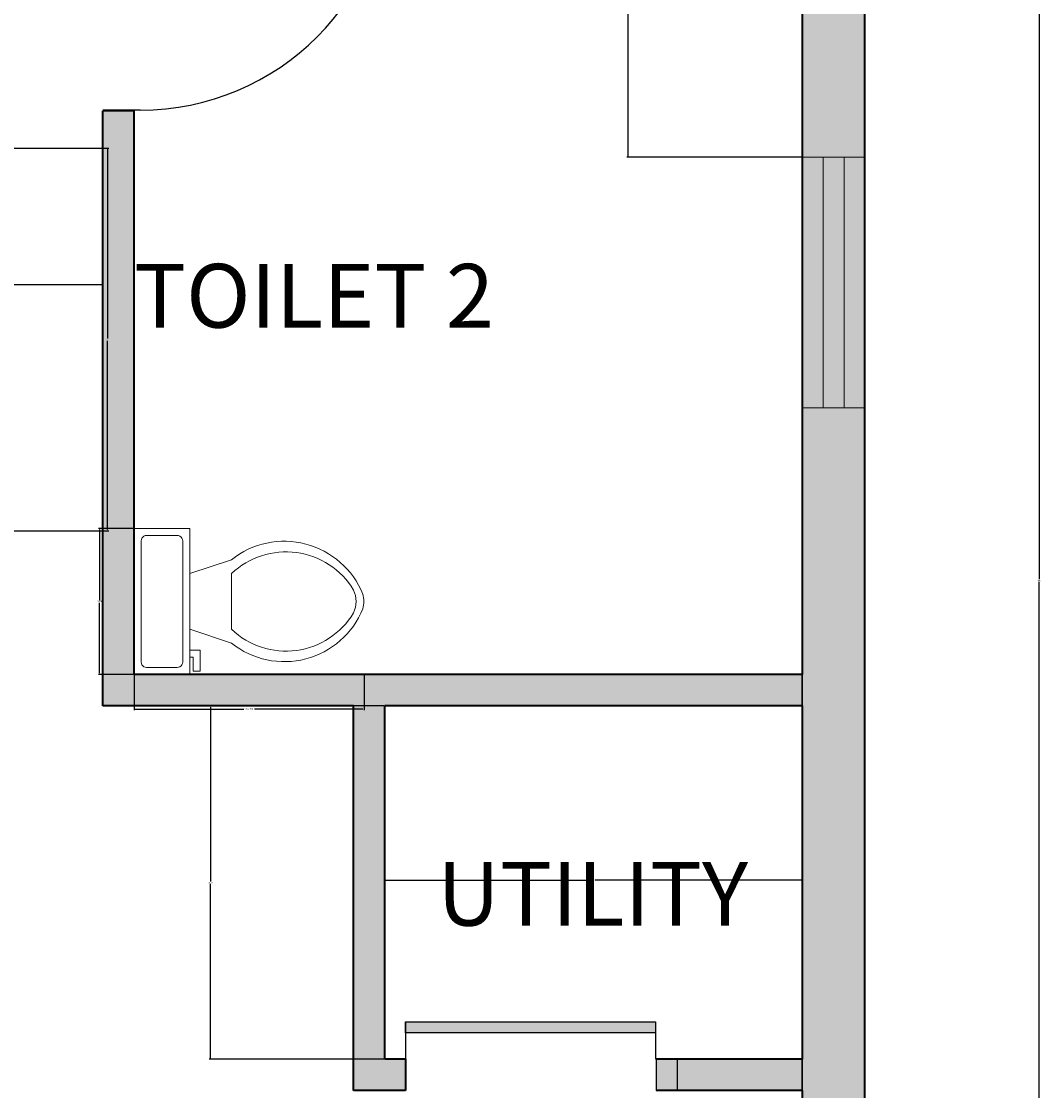
# Model space of a CAD drawing. Units: inches. Extents: x 1434 to 1845, y 1483 to 2014.
# Tile 8 of 11: x 1698 to 1845, y 1675 to 1829. Entities that reach past the tile are written whole.
import ezdxf

# ---------------------------------------------------------------- set-up
doc = ezdxf.new("R2010")
doc.units = ezdxf.units.IN
for name, color, linetype, lineweight in [('A-ANNO-DIMS', 2, 'Continuous', 18), ('A-AREA-IDEN', 7, 'Continuous', 25), ('A-DOOR', 3, 'Continuous', 25), ('A-FLOR-FIXT', 8, 'Continuous', 18), ('A-GLAZ', 4, 'Continuous', 18), ('A-GLAZ-PATT', 9, 'Continuous', 13), ('A-WALL', 7, 'Continuous', 35), ('A-WALL-PATT', 8, 'Continuous', 13)]:
    doc.layers.add(name, color=color, linetype=linetype, lineweight=lineweight)
doc.layers.add('A-DOOR-PATT', color=39, linetype='Continuous', lineweight=13, true_color=0x58382b)
doc.styles.get("Standard").update_dxf_attribs({"font": 'arial.ttf'})
doc.dimstyles.get("Standard").update_dxf_attribs({"dimtxt": 0.18, "dimasz": 0.18, "dimexe": 0.18, "dimexo": 0.0625, "dimgap": 0.09, "dimtad": 0, "dimtih": 1, "dimtoh": 1, "dimdec": 4, "dimzin": 0, "dimdsep": 46, "dimtxsty": 'Standard', "dimcen": 0.09, "dimadec": 0, "dimazin": 0, "dimtfac": 1, "dimtdec": 4, "dimtofl": 0, "dimtmove": 0, "dimatfit": 3, "dimfxl": 1, "dimtolj": 1, "dimtzin": 0, "dimarcsym": 0})

# ---------------------------------------------------------------- blocks, each defined once
blk = doc.blocks.new('*U3')
for p, q in [((0, 0), (0, -6)), ((40, 0), (40, -6))]:
    blk.add_line(p, q)
blk.add_lwpolyline([(0, 0), (0, 40), (1.75, 40), (1.75, 0)], close=True)
blk.add_arc((0, 0), 40, 0, 90)
blk = doc.blocks.new('*U5')
for p, q in [((0, 0), (0, -6)), ((40, 0), (40, -6))]:
    blk.add_line(p, q)
blk.add_lwpolyline([(0, 0), (40, 0), (40, -1.75), (0, -1.75)], close=True)
blk = doc.blocks.new('Toilet - top')
for p, q in [((9.5, -6), (9.5, -2)), ((-10, -8.5), (-8, -8.5)), ((-10, -9.5), (-10, -8.5)), ((-8, -8.5), (-8, -8)), ((-7, -8), (-7, -9.5)), ((-4, -8), (-6, -14)), ((4, -8), (6, -14)), ((-7, -9.5), (-10, -9.5)), ((4, -14), (-4, -14))]:
    blk.add_line(p, q)
blk.add_lwpolyline([(10.5, -8), (10.5, 0), (-10.5, 0), (-10.5, -8)], close=True)
for points in [[(8.5, -1), (-8.5, -1)], [(-9.5, -2), (-9.5, -6)], [(-8.5, -7), (8.5, -7)]]:
    blk.add_lwpolyline(points)
for centre, radius, start, end in [((-8.62, -1.88), 0.884, 81.8699, 188.1301), ((8.62, -1.88), 0.884, 351.8699, 98.1301), ((-8.62, -6.12), 0.884, 171.8699, 278.1301), ((8.62, -6.12), 0.884, 261.8699, 8.1301), ((3.52, -21.58), 12.17, 141.4691, 247.9714), ((4.2, -21.82), 11.33, 136.3677, 238.9468), ((-3.52, -21.58), 12.17, 292.0284, 38.5307), ((-4.2, -21.82), 11.33, 301.053, 43.6321), ((0, -27.88), 4, 245.7318, 294.2682), ((0, -29), 4, 254.8605, 285.1395)]:
    blk.add_arc(centre, radius, start, end)
blk = doc.blocks.new('WIN-36IN-9IN')
for p, q in [((3, 36), (3, 0)), ((6, 36), (6, 0))]:
    blk.add_line(p, q)
blk.add_lwpolyline([(9, 0), (9, 36), (0, 36), (0, 0)], close=True)
blk = doc.blocks.new('*D36')
at = {"layer": 'A-ANNO-DIMS', "color": 0, "lineweight": -2, "transparency": 16777216}
for p, q in [((1714.47, 1734.79), (1714.47, 1729.72)), ((1747.52, 1734.79), (1747.52, 1729.72)), ((1714.65, 1729.9), (1730.22, 1729.9)), ((1747.34, 1729.9), (1731.77, 1729.9))]:
    blk.add_line(p, q, dxfattribs=at)
at = {"layer": 'A-ANNO-DIMS', "color": 0, "transparency": 16777216}
for points in [[(1714.65, 1729.93), (1714.65, 1729.87), (1714.47, 1729.9)], [(1747.34, 1729.93), (1747.34, 1729.87), (1747.52, 1729.9)]]:
    blk.add_solid(points, dxfattribs=at)
at = {"layer": 'Defpoints', "color": 0, "transparency": 16777216}
for p in [(1714.47, 1734.86), (1747.52, 1734.86), (1714.47, 1729.9)]:
    blk.add_point(p, dxfattribs=at)
at = {"layer": 'A-ANNO-DIMS', "color": 0, "transparency": 16777216, "insert": (1731, 1729.9), "char_height": 0.18, "attachment_point": 5}
blk.add_mtext('\\A1;WC 33 TYP.', dxfattribs=at)
blk = doc.blocks.new('*D37')
at = {"layer": 'A-ANNO-DIMS', "color": 0, "lineweight": -2, "transparency": 16777216}
for p, q in [((1714.41, 1755.86), (1709.34, 1755.86)), ((1709.52, 1755.68), (1709.52, 1745.54)), ((1709.52, 1735.04), (1709.52, 1745.17)), ((1714.41, 1734.86), (1709.34, 1734.86))]:
    blk.add_line(p, q, dxfattribs=at)
at = {"layer": 'A-ANNO-DIMS', "color": 0, "transparency": 16777216}
for points in [[(1709.49, 1755.68), (1709.55, 1755.68), (1709.52, 1755.86)], [(1709.49, 1735.04), (1709.55, 1735.04), (1709.52, 1734.86)]]:
    blk.add_solid(points, dxfattribs=at)
at = {"layer": 'Defpoints', "color": 0, "transparency": 16777216}
for p in [(1709.52, 1755.86), (1714.47, 1755.86), (1714.47, 1734.86)]:
    blk.add_point(p, dxfattribs=at)
at = {"layer": 'A-ANNO-DIMS', "color": 0, "transparency": 16777216, "insert": (1709.52, 1745.36), "char_height": 0.18, "attachment_point": 5}
blk.add_mtext('\\A1;21 TYP.', dxfattribs=at)
blk = doc.blocks.new('*D43')
at = {"layer": 'A-ANNO-DIMS', "color": 0, "lineweight": -2, "transparency": 16777216}
for p, q in [((1697.08, 1810.5), (1710.85, 1810.5)), ((1710.67, 1810.32), (1710.67, 1783.19)), ((1710.67, 1755.68), (1710.67, 1782.82)), ((1697.08, 1755.5), (1710.85, 1755.5))]:
    blk.add_line(p, q, dxfattribs=at)
at = {"layer": 'A-ANNO-DIMS', "color": 0, "transparency": 16777216}
for points in [[(1710.64, 1810.32), (1710.7, 1810.32), (1710.67, 1810.5)], [(1710.64, 1755.68), (1710.7, 1755.68), (1710.67, 1755.5)]]:
    blk.add_solid(points, dxfattribs=at)
at = {"layer": 'Defpoints', "color": 0, "transparency": 16777216}
for p in [(1697.02, 1810.5), (1710.67, 1810.5), (1697.02, 1755.5)]:
    blk.add_point(p, dxfattribs=at)
at = {"layer": 'A-ANNO-DIMS', "color": 0, "transparency": 16777216, "insert": (1710.67, 1783), "char_height": 0.18, "attachment_point": 5}
blk.add_mtext('\\A1;55', dxfattribs=at)
blk = doc.blocks.new('*D55')
at = {"layer": 'A-ANNO-DIMS', "color": 0, "lineweight": -2, "transparency": 16777216}
for p, q in [((1819.54, 1988.36), (1844.68, 1988.36)), ((1844.5, 1988.18), (1844.5, 1748.54)), ((1844.5, 1508.54), (1844.5, 1748.17)), ((1819.54, 1508.36), (1844.68, 1508.36))]:
    blk.add_line(p, q, dxfattribs=at)
at = {"layer": 'A-ANNO-DIMS', "color": 0, "transparency": 16777216}
for points in [[(1844.47, 1988.18), (1844.53, 1988.18), (1844.5, 1988.36)], [(1844.47, 1508.54), (1844.53, 1508.54), (1844.5, 1508.36)]]:
    blk.add_solid(points, dxfattribs=at)
at = {"layer": 'Defpoints', "color": 0, "transparency": 16777216}
for p in [(1819.47, 1988.36), (1844.5, 1988.36), (1819.47, 1508.36)]:
    blk.add_point(p, dxfattribs=at)
at = {"layer": 'A-ANNO-DIMS', "color": 0, "transparency": 16777216, "insert": (1844.5, 1748.36), "char_height": 0.18, "attachment_point": 5}
blk.add_mtext('\\A1;480', dxfattribs=at)
blk = doc.blocks.new('*D58')
at = {"layer": 'A-ANNO-DIMS', "color": 0, "lineweight": -2, "transparency": 16777216}
for p, q in [((1670.97, 1974.79), (1670.97, 1483.15)), ((1810.47, 1974.79), (1810.47, 1483.15)), ((1671.15, 1483.33), (1740.34, 1483.33)), ((1810.29, 1483.33), (1741.11, 1483.33))]:
    blk.add_line(p, q, dxfattribs=at)
at = {"layer": 'A-ANNO-DIMS', "color": 0, "transparency": 16777216}
for points in [[(1671.15, 1483.36), (1671.15, 1483.3), (1670.97, 1483.33)], [(1810.29, 1483.36), (1810.29, 1483.3), (1810.47, 1483.33)]]:
    blk.add_solid(points, dxfattribs=at)
at = {"layer": 'Defpoints', "color": 0, "transparency": 16777216}
for p in [(1670.97, 1974.86), (1810.47, 1974.86), (1810.47, 1483.33)]:
    blk.add_point(p, dxfattribs=at)
at = {"layer": 'A-ANNO-DIMS', "color": 0, "transparency": 16777216, "insert": (1740.72, 1483.33), "char_height": 0.18, "attachment_point": 5}
blk.add_mtext('\\A1;139.5', dxfattribs=at)
blk = doc.blocks.new('*D62')
at = {"layer": 'A-ANNO-DIMS', "color": 0, "lineweight": -2, "transparency": 16777216}
for p, q in [((1573.47, 1815.79), (1573.47, 1790.65)), ((1709.97, 1815.79), (1709.97, 1790.65)), ((1573.65, 1790.83), (1641.34, 1790.83)), ((1709.79, 1790.83), (1642.11, 1790.83))]:
    blk.add_line(p, q, dxfattribs=at)
at = {"layer": 'A-ANNO-DIMS', "color": 0, "transparency": 16777216}
for points in [[(1573.65, 1790.86), (1573.65, 1790.8), (1573.47, 1790.83)], [(1709.79, 1790.86), (1709.79, 1790.8), (1709.97, 1790.83)]]:
    blk.add_solid(points, dxfattribs=at)
at = {"layer": 'Defpoints', "color": 0, "transparency": 16777216}
for p in [(1573.47, 1815.86), (1709.97, 1815.86), (1573.47, 1790.83)]:
    blk.add_point(p, dxfattribs=at)
at = {"layer": 'A-ANNO-DIMS', "color": 0, "transparency": 16777216, "insert": (1641.72, 1790.83), "char_height": 0.18, "attachment_point": 5}
blk.add_mtext('\\A1;136.5', dxfattribs=at)
blk = doc.blocks.new('*D67')
at = {"layer": 'A-ANNO-DIMS', "color": 0, "lineweight": -2, "transparency": 16777216}
for p, q in [((1694.97, 1517.42), (1694.97, 2013.56)), ((1695.15, 2013.38), (1752.34, 2013.38)), ((1810.29, 2013.38), (1753.11, 2013.38)), ((1810.47, 1517.42), (1810.47, 2013.56))]:
    blk.add_line(p, q, dxfattribs=at)
at = {"layer": 'A-ANNO-DIMS', "color": 0, "transparency": 16777216}
for points in [[(1695.15, 2013.41), (1695.15, 2013.35), (1694.97, 2013.38)], [(1810.29, 2013.41), (1810.29, 2013.35), (1810.47, 2013.38)]]:
    blk.add_solid(points, dxfattribs=at)
at = {"layer": 'Defpoints', "color": 0, "transparency": 16777216}
for p in [(1810.47, 2013.38), (1694.97, 1517.36), (1810.47, 1517.36)]:
    blk.add_point(p, dxfattribs=at)
at = {"layer": 'A-ANNO-DIMS', "color": 0, "transparency": 16777216, "insert": (1752.72, 2013.38), "char_height": 0.18, "attachment_point": 5}
blk.add_mtext('\\A1;115.5', dxfattribs=at)
blk = doc.blocks.new('*D68')
at = {"layer": 'A-ANNO-DIMS', "color": 0, "lineweight": -2, "transparency": 16777216}
for p, q in [((1750.47, 1730.29), (1750.47, 1705.15)), ((1810.47, 1730.29), (1810.47, 1705.15)), ((1750.65, 1705.33), (1780.26, 1705.33)), ((1810.29, 1705.33), (1780.69, 1705.33))]:
    blk.add_line(p, q, dxfattribs=at)
at = {"layer": 'A-ANNO-DIMS', "color": 0, "transparency": 16777216}
for points in [[(1750.65, 1705.36), (1750.65, 1705.3), (1750.47, 1705.33)], [(1810.29, 1705.36), (1810.29, 1705.3), (1810.47, 1705.33)]]:
    blk.add_solid(points, dxfattribs=at)
at = {"layer": 'Defpoints', "color": 0, "transparency": 16777216}
for p in [(1750.47, 1730.36), (1810.47, 1730.36), (1750.47, 1705.33)]:
    blk.add_point(p, dxfattribs=at)
at = {"layer": 'A-ANNO-DIMS', "color": 0, "transparency": 16777216, "insert": (1780.47, 1705.33), "char_height": 0.18, "attachment_point": 5}
blk.add_mtext('\\A1;60', dxfattribs=at)
blk = doc.blocks.new('*D69')
at = {"layer": 'A-ANNO-DIMS', "color": 0, "lineweight": -2, "transparency": 16777216}
for p, q in [((1750.41, 1730.36), (1725.27, 1730.36)), ((1725.45, 1730.18), (1725.45, 1705.15)), ((1725.45, 1679.76), (1725.45, 1704.79)), ((1750.41, 1679.58), (1725.27, 1679.58))]:
    blk.add_line(p, q, dxfattribs=at)
at = {"layer": 'A-ANNO-DIMS', "color": 0, "transparency": 16777216}
for points in [[(1725.42, 1730.18), (1725.48, 1730.18), (1725.45, 1730.36)], [(1725.42, 1679.76), (1725.48, 1679.76), (1725.45, 1679.58)]]:
    blk.add_solid(points, dxfattribs=at)
at = {"layer": 'Defpoints', "color": 0, "transparency": 16777216}
for p in [(1725.45, 1730.36), (1750.47, 1730.36), (1750.47, 1679.58)]:
    blk.add_point(p, dxfattribs=at)
at = {"layer": 'A-ANNO-DIMS', "color": 0, "transparency": 16777216, "insert": (1725.45, 1704.97), "char_height": 0.18, "attachment_point": 5}
blk.add_mtext('\\A1;50.77', dxfattribs=at)
blk = doc.blocks.new('*D79')
at = {"layer": 'A-ANNO-DIMS', "color": 0, "lineweight": -2, "transparency": 16777216}
for p, q in [((1810.41, 1854.86), (1785.27, 1854.86)), ((1785.45, 1854.68), (1785.45, 1832.19)), ((1785.45, 1809.35), (1785.45, 1831.83)), ((1810.41, 1809.17), (1785.27, 1809.17))]:
    blk.add_line(p, q, dxfattribs=at)
at = {"layer": 'A-ANNO-DIMS', "color": 0, "transparency": 16777216}
for points in [[(1785.42, 1854.68), (1785.48, 1854.68), (1785.45, 1854.86)], [(1785.42, 1809.35), (1785.48, 1809.35), (1785.45, 1809.17)]]:
    blk.add_solid(points, dxfattribs=at)
at = {"layer": 'Defpoints', "color": 0, "transparency": 16777216}
for p in [(1785.45, 1854.86), (1810.47, 1854.86), (1810.47, 1809.17)]:
    blk.add_point(p, dxfattribs=at)
at = {"layer": 'A-ANNO-DIMS', "color": 0, "transparency": 16777216, "insert": (1785.45, 1832.01), "char_height": 0.18, "attachment_point": 5}
blk.add_mtext('\\A1;45.69', dxfattribs=at)

msp = doc.modelspace()

# ---------------------------------------------------------------- hatches: boundary and pattern name
at = {"layer": 'A-DOOR-PATT'}
h = msp.add_hatch(color=256, dxfattribs=at)
h.dxf.hatch_style = 1
h.paths.add_polyline_path([(1611.5864, 1583.2737), (1575.6681, 1583.2737, 0.01094143), (1575.7025, 1581.7022), (1611.5864, 1581.7022)])
h.paths.add_polyline_path([(1621.4742, 1547.3553), (1616.9742, 1547.3553), (1616.9742, 1544.3553), (1621.4742, 1544.3553)])
h.paths.add_polyline_path([(1635.0456, 1558.627, 0.01094143), (1633.4742, 1558.6614), (1633.4742, 1522.7431), (1635.0456, 1522.7431)])
h.paths.add_polyline_path([(1633.4742, 1517.3553), (1630.4742, 1517.3553), (1630.4742, 1508.3553), (1633.4742, 1508.3553)])
h.paths.add_polyline_path([(1672.8212, 1517.3553), (1669.8212, 1517.3553), (1669.8212, 1508.3553), (1672.8212, 1508.3553)])
h.paths.add_polyline_path([(1613.8925, 1724.9676), (1612.3211, 1724.9676), (1612.3211, 1689.0836, 0.01094143), (1613.8925, 1689.0492)])
h.paths.add_polyline_path([(1789.3925, 1684.9726), (1753.4742, 1684.9726), (1753.4742, 1683.4011), (1789.3925, 1683.4011)])
h.paths.add_polyline_path([(1792.4742, 1679.5848), (1789.4742, 1679.5848), (1789.4742, 1675.0848), (1792.4742, 1675.0848)])
h.paths.add_polyline_path([(1563.5864, 1851.7737), (1527.6681, 1851.7737, 0.01094143), (1527.7025, 1850.2022), (1563.5864, 1850.2022)])
h.paths.add_polyline_path([(1609.3925, 1900.6614, 0.01094143), (1607.8211, 1900.627), (1607.8211, 1864.7431), (1609.3925, 1864.7431)])
h.paths.add_polyline_path([(1675.5456, 1900.627, 0.01094143), (1673.9742, 1900.6614), (1673.9742, 1864.7431), (1675.5456, 1864.7431)])
h.paths.add_polyline_path([(1751.2803, 1851.8553), (1715.3619, 1851.8553), (1715.3619, 1850.2839), (1751.2459, 1850.2839, 0.01094143)])
at = {"layer": 'A-GLAZ-PATT'}
h = msp.add_hatch(color=256, dxfattribs=at)
h.dxf.hatch_style = 1
h.set_gradient(color1=(0, 0, 255), color2=(255, 255, 0), name='INVSPHERICAL')
h.paths.add_polyline_path([(1819.4742, 1809.1667), (1816.4742, 1809.1667), (1816.4742, 1773.1667), (1819.4742, 1773.1667)])
h.paths.add_polyline_path([(1816.4742, 1809.1667), (1813.4742, 1809.1667), (1813.4742, 1773.1667), (1816.4742, 1773.1667)])
h.paths.add_polyline_path([(1813.4742, 1809.1667), (1810.4742, 1809.1667), (1810.4742, 1773.1667), (1813.4742, 1773.1667)])
at = {"layer": 'A-WALL-PATT'}
h = msp.add_hatch(color=256, dxfattribs=at)
h.dxf.hatch_style = 1
h.paths.add_polyline_path([(1472.9742, 1730.3553), (1577.9742, 1730.3553), (1577.9742, 1734.8553), (1573.4742, 1734.8553), (1573.4742, 1815.8553), (1568.9742, 1815.8553), (1568.9742, 1734.8553), (1472.9742, 1734.8553), (1472.9742, 1770.1951), (1459.9742, 1770.1951), (1459.9742, 1782.1951), (1459.9742, 1818.1951), (1472.9742, 1818.1951), (1472.9742, 1854.8553), (1568.9742, 1854.8553), (1568.9742, 1851.8553), (1573.4742, 1851.8553), (1573.4742, 1854.8553), (1573.4742, 1859.3553), (1472.9742, 1859.3553), (1472.9742, 1899.9369), (1459.9742, 1899.9369), (1459.9742, 1911.9369), (1459.9742, 1947.9369), (1472.9742, 1947.9369), (1472.9742, 1974.8553), (1513.9785, 1974.8553), (1513.9785, 1987.8553), (1561.9785, 1987.8553), (1561.9785, 1974.8553), (1612.4742, 1974.8553), (1612.4742, 1859.3553), (1609.4742, 1859.3553), (1609.4742, 1854.8553), (1616.9742, 1854.8553), (1616.9742, 1910.3553), (1625.153, 1910.3553), (1625.153, 1914.8553), (1616.9742, 1914.8553), (1616.9742, 1988.3553), (1459.4742, 1988.3553), (1459.4742, 1508.3553), (1630.4742, 1508.3553), (1630.4742, 1517.3553), (1472.9742, 1517.3553), (1472.9742, 1586.3553), (1616.9742, 1586.3553), (1616.9742, 1583.3553), (1621.4742, 1583.3553), (1621.4742, 1586.3553), (1621.4742, 1734.8553), (1616.9742, 1734.8553), (1613.9742, 1734.8553), (1613.9742, 1730.3553), (1616.9742, 1730.3553), (1616.9742, 1590.8553), (1472.9742, 1590.8553), (1472.9742, 1635.7299), (1459.9742, 1635.7299), (1459.9742, 1647.7299), (1459.9742, 1683.7299), (1472.9742, 1683.7299)])
h.paths.add_polyline_path([(1819.4742, 1773.1667), (1810.4742, 1773.1667), (1810.4742, 1734.8553), (1714.4742, 1734.8553), (1714.4742, 1815.8553), (1709.9742, 1815.8553), (1709.9742, 1730.3553), (1745.9742, 1730.3553), (1745.9742, 1675.0848), (1753.4742, 1675.0848), (1753.4742, 1679.5848), (1750.4742, 1679.5848), (1750.4742, 1730.3553), (1810.4742, 1730.3553), (1810.4742, 1679.5848), (1792.4742, 1679.5848), (1792.4742, 1675.0848), (1810.4742, 1675.0848), (1810.4742, 1517.3553), (1775.1129, 1517.3553), (1775.1129, 1508.3553), (1819.4742, 1508.3553)])
h.paths.add_polyline_path([(1739.1129, 1517.3553), (1694.9742, 1517.3553), (1694.9742, 1730.3553), (1690.4742, 1730.3553), (1690.4742, 1517.3553), (1678.4742, 1517.3553), (1675.4742, 1517.3553), (1672.8212, 1517.3553), (1672.8212, 1508.3553), (1678.4742, 1508.3553), (1739.1129, 1508.3553)])
h.paths.add_polyline_path([(1735.6549, 1987.8553), (1783.6549, 1987.8553), (1783.6549, 1974.8553), (1810.4742, 1974.8553), (1810.4742, 1859.3553), (1709.9742, 1859.3553), (1709.9742, 1854.8553), (1709.9742, 1851.8553), (1714.4742, 1851.8553), (1714.4742, 1854.8553), (1810.4742, 1854.8553), (1810.4742, 1809.1667), (1819.4742, 1809.1667), (1819.4742, 1988.3553), (1666.4742, 1988.3553), (1666.4742, 1914.8553), (1661.1087, 1914.8553), (1661.1087, 1910.3553), (1666.4742, 1910.3553), (1666.4742, 1854.8553), (1673.9742, 1854.8553), (1673.9742, 1859.3553), (1670.9742, 1859.3553), (1670.9742, 1974.8553), (1735.6549, 1974.8553)])

# ---------------------------------------------------------------- linework, layer by layer
at = {"layer": 'A-DOOR'}
for p, q in [((1789.4742, 1679.5848), (1789.4742, 1675.0848)), ((1792.4742, 1679.5848), (1792.4742, 1675.0848))]:
    msp.add_line(p, q, dxfattribs=at)
at = {"layer": 'A-WALL'}
for p, q in [((1810.4742, 1734.8553), (1810.4742, 1854.8553)), ((1709.9742, 1730.3553), (1709.9742, 1815.8553)), ((1714.4742, 1815.8553), (1709.9742, 1815.8553)), ((1714.4742, 1734.8553), (1714.4742, 1815.8553)), ((1810.4742, 1734.8553), (1714.4742, 1734.8553)), ((1745.9742, 1730.3553), (1709.9742, 1730.3553)), ((1745.9742, 1675.0848), (1745.9742, 1730.3553)), ((1810.4742, 1730.3553), (1750.4742, 1730.3553)), ((1750.4742, 1679.5848), (1750.4742, 1730.3553)), ((1810.4742, 1679.5848), (1810.4742, 1730.3553)), ((1753.4742, 1679.5848), (1750.4742, 1679.5848)), ((1753.4742, 1679.5848), (1753.4742, 1675.0848)), ((1810.4742, 1679.5848), (1789.4742, 1679.5848)), ((1753.4742, 1675.0848), (1745.9742, 1675.0848)), ((1810.4742, 1675.0848), (1789.4742, 1675.0848)), ((1810.4742, 1517.3553), (1810.4742, 1675.0848))]:
    msp.add_line(p, q, dxfattribs=at)
msp.add_lwpolyline([(1678.4742, 1508.3553), (1819.4742, 1508.3553), (1819.4742, 1988.3553), (1459.4742, 1988.3553), (1459.4742, 1508.3553), (1630.4742, 1508.3553)], dxfattribs=at)

# ---------------------------------------------------------------- block references
at = {"layer": 'A-DOOR', "xscale": 0.8979587755198419, "yscale": 0.8979587755198419, "zscale": 0.8979587755198419, "rotation": 270}
msp.add_blockref('*U3', (1715.3619, 1851.8553), dxfattribs=at)
at = {"layer": 'A-DOOR', "xscale": 0.8979587755198419, "yscale": 0.8979587755198419, "zscale": 0.8979587755198419}
msp.add_blockref('*U5', (1753.4742, 1684.9726), dxfattribs=at)
at = {"layer": 'A-FLOR-FIXT', "rotation": 90}
msp.add_blockref('Toilet - top', (1714.4742, 1745.3553), dxfattribs=at)
at = {"layer": 'A-GLAZ'}
msp.add_blockref('WIN-36IN-9IN', (1810.4742, 1773.1667), dxfattribs=at)

# ---------------------------------------------------------------- texts
at = {"layer": 'A-AREA-IDEN'}
for s, p in [('TOILET 2 ', (1714.4742, 1784.6994)), ('UTILITY', (1758.0276, 1698.7815))]:
    msp.add_text(s, height=9.14668, dxfattribs=at).set_placement(p)

# ---------------------------------------------------------------- dimensions: what is measured, and where the dimension line sits
at = {"layer": 'A-ANNO-DIMS'}
for base, p1, p2, picture, middle in [((1810.4742, 2013.3803), (1694.9742, 1517.3553), (1810.4742, 1517.3553), '*D67', (1752.7242, 2013.3803)), ((1810.4742, 1483.3303), (1670.9742, 1974.8553), (1810.4742, 1974.8553), '*D58', (1740.7242, 1483.3303))]:
    dim = msp.add_linear_dim(base=base, p1=p1, p2=p2, dimstyle='Standard', override={"dimdec": 1, "dimlfac": 1, "dimrnd": 0, "dimzin": 0, "dimdsep": 46, "dimlunit": 2}, dxfattribs=at)
    dim.commit()
    dim.dimension.update_dxf_attribs({"geometry": picture, "text_midpoint": middle})
for base, p1, p2, angle, override, picture, middle in [((1844.4992, 1988.3553), (1819.4742, 1508.3553), (1819.4742, 1988.3553), 90, {"dimdec": 0, "dimlfac": 1, "dimrnd": 0, "dimzin": 0, "dimdsep": 46, "dimlunit": 2}, '*D55', (1844.4992, 1748.3553)), ((1785.4492, 1854.8553), (1810.4742, 1809.1667), (1810.4742, 1854.8553), 90, {"dimdec": 2, "dimlfac": 1, "dimrnd": 0, "dimzin": 0, "dimdsep": 46, "dimlunit": 2}, '*D79', (1785.4492, 1832.011)), ((1573.4742, 1790.8303), (1709.9742, 1815.8553), (1573.4742, 1815.8553), 180, {"dimdec": 1, "dimlfac": 1, "dimrnd": 0, "dimzin": 0, "dimdsep": 46, "dimlunit": 2}, '*D62', (1641.7242, 1790.8303)), ((1710.6673, 1810.5049), (1697.0173, 1755.5049), (1697.0173, 1810.5049), 90, {"dimdec": 0, "dimlfac": 1, "dimrnd": 0, "dimzin": 0, "dimdsep": 46, "dimlunit": 2}, '*D43', (1710.6673, 1783.0049)), ((1725.4492, 1730.3553), (1750.4742, 1679.5848), (1750.4742, 1730.3553), 90, {"dimdec": 2, "dimlfac": 1, "dimrnd": 0, "dimzin": 0, "dimdsep": 46, "dimlunit": 2}, '*D69', (1725.4492, 1704.9701)), ((1750.4742, 1705.3303), (1810.4742, 1730.3553), (1750.4742, 1730.3553), 180, {"dimdec": 0, "dimlfac": 1, "dimrnd": 0, "dimzin": 0, "dimdsep": 46, "dimlunit": 2}, '*D68', (1780.4742, 1705.3303))]:
    dim = msp.add_linear_dim(base=base, p1=p1, p2=p2, angle=angle, dimstyle='Standard', override=override, dxfattribs=at)
    dim.commit()
    dim.dimension.update_dxf_attribs({"geometry": picture, "text_midpoint": middle})
for base, p1, p2, angle, text, picture, middle in [((1709.5173, 1755.8553), (1714.4742, 1734.8553), (1714.4742, 1755.8553), 90, '<> TYP.', '*D37', (1709.5173, 1745.3553)), ((1714.4742, 1729.8984), (1747.5204, 1734.8553), (1714.4742, 1734.8553), 180, 'WC <> TYP.', '*D36', (1730.9973, 1729.8984))]:
    dim = msp.add_linear_dim(base=base, p1=p1, p2=p2, angle=angle, text=text, dimstyle='Standard', override={"dimdec": 0, "dimlfac": 1, "dimrnd": 0, "dimzin": 0, "dimdsep": 46, "dimlunit": 2}, dxfattribs=at)
    dim.commit()
    dim.dimension.update_dxf_attribs({"geometry": picture, "text_midpoint": middle})

doc.saveas('drawing.dxf')
